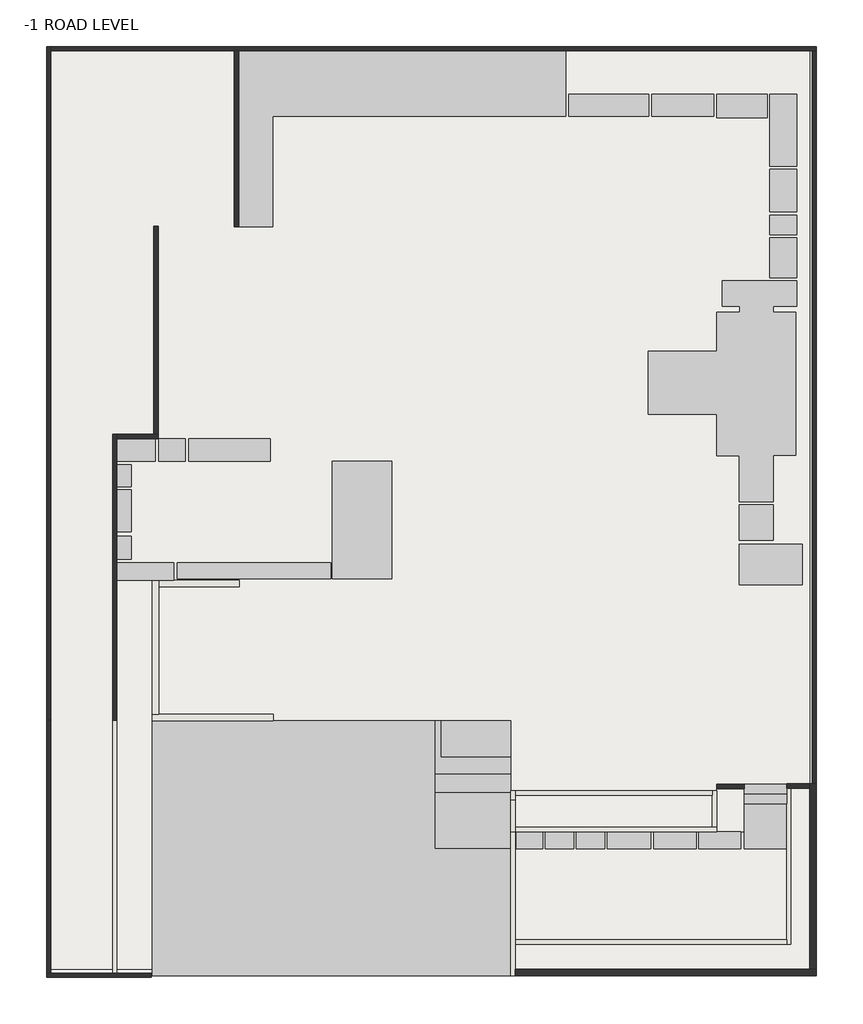
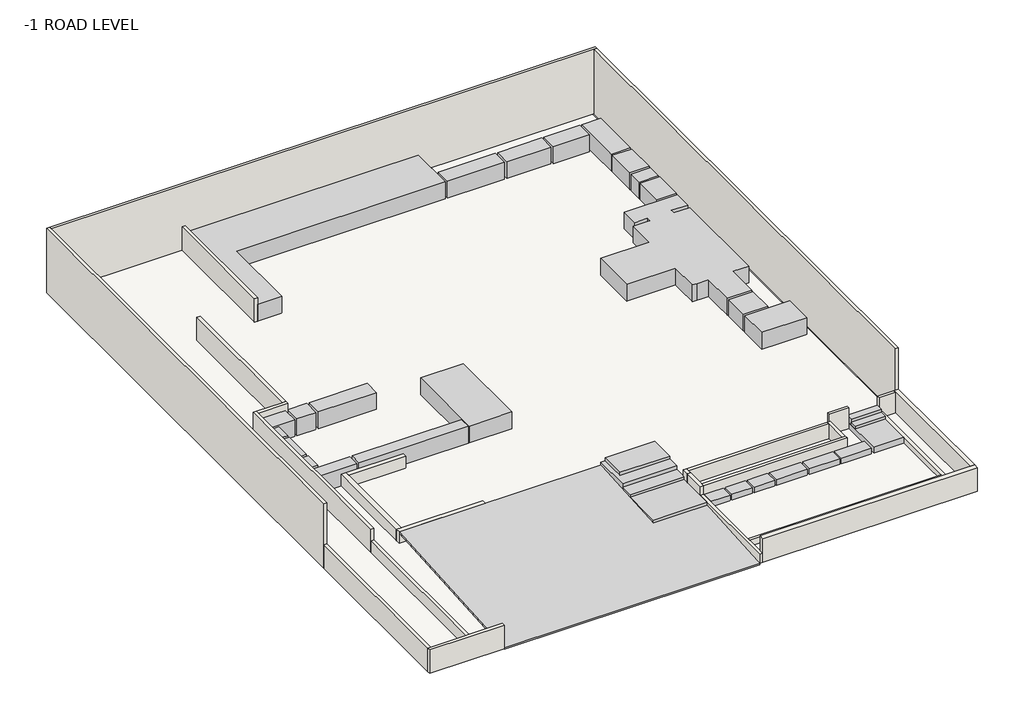
# One storey: 25 walls, 2 proxies, 2 slabs, 1 ramp.
"""IFC4 building model written with IfcOpenShell, lengths in millimetres."""

from ifc_helpers import new_model, si_unit, frame, origin, place, context, project, spatial, polyline, outline, extrude, faceted_brep, transform, mapped, element, save
from components import generic_models_1_generic_models_1_8db9de98, generic_models_2_generic_models_2_cbc3407a, ramp_2_3d1851f7

model = new_model("IFC4")

# Units and contexts
model_context = context("Model", 3, world=origin())
ifc_project = project(units=[si_unit("LENGTHUNIT", "METRE", prefix="MILLI")], contexts=[model_context])

# Site, building, storey
site = spatial("IfcSite", under=ifc_project)
building = spatial("IfcBuilding", under=site)
storey = spatial("IfcBuildingStorey", under=building, Name="-1 ROAD LEVEL", Elevation=-914.4)

# Proxies
placement = place(None, origin())
generic_models_1_generic_models_1_shape = generic_models_1_generic_models_1_8db9de98(model_context)
element("IfcBuildingElementProxy", 1, Name="Generic Models 1 : Generic Models 1", ObjectType="Generic Models 1 : Generic Models 1", at=placement, inside=storey, context=model_context, shape_type="MappedRepresentation", body=[
    mapped(generic_models_1_generic_models_1_shape, transform((0.0, 0.0, 0.0), x_axis=(1.0, 0.0, 0.0), y_axis=(0.0, 1.0, 0.0), z_axis=(0.0, 0.0, 1.0))),
])
generic_models_2_generic_models_2_shape = generic_models_2_generic_models_2_cbc3407a(model_context)
element("IfcBuildingElementProxy", 2, Name="Generic Models 2 : Generic Models 2", ObjectType="Generic Models 2 : Generic Models 2", at=placement, inside=storey, context=model_context, shape_type="MappedRepresentation", body=[
    mapped(generic_models_2_generic_models_2_shape, transform((0.0, 0.0, 0.0), x_axis=(1.0, 0.0, 0.0), y_axis=(0.0, 1.0, 0.0), z_axis=(0.0, 0.0, 1.0))),
])

# Ramp
ramp_2_shape = ramp_2_3d1851f7(model_context)
element("IfcRamp", 3, ObjectType="Ramp 2", at=placement, inside=storey, context=model_context, shape_type="MappedRepresentation", body=[
    mapped(ramp_2_shape, transform((0.0, 0.0, 0.0), x_axis=(1.0, 0.0, 0.0), y_axis=(0.0, 1.0, 0.0), z_axis=(0.0, 0.0, 1.0))),
])

# Slabs
element("IfcSlab", 4, ObjectType="6\"", at=placement, inside=storey, context=model_context, shape_type="SweptSolid", body=[
    extrude(outline(polyline([(7185.8179176, -9972.5794723), (7185.8179176, -11102.8794723), (282.0588295, -11102.8794723), (282.0588295, -9972.5794723), (7185.8179176, -9972.5794723)])), frame((0.0, 0.0, -914.4), z_axis=(0.0, 0.0, 1.0), x_axis=(1.0, 0.0, 0.0)), (0.0, 0.0, 1.0), 152.4),
    extrude(outline(polyline([(8295.7588295, -9743.9794723), (8295.7588295, -11255.2794723), (7338.2179176, -11255.2794723), (7338.2179176, -9743.9794723), (8295.7588295, -9743.9794723)])), frame((0.0, 0.0, -914.4), z_axis=(0.0, 0.0, 1.0), x_axis=(1.0, 0.0, 0.0)), (0.0, 0.0, 1.0), 152.4),
    extrude(outline(polyline([(10594.4588295, -9735.0018845), (10594.4588295, -16072.3018845), (9934.0588295, -16072.3018845), (282.0588295, -16072.3018845), (282.0588295, -15196.0018845), (9934.0588295, -15196.0018845), (9934.0588295, -9735.0018845), (10594.4588295, -9735.0018845)])), frame((0.0, 0.0, -914.4), z_axis=(0.0, 0.0, 1.0), x_axis=(1.0, 0.0, 0.0)), (0.0, 0.0, 1.0), 152.4),
    extrude(outline(polyline([(9781.6588295, -11267.9794723), (9781.6588295, -15043.6018845), (282.0588295, -15043.6018845), (282.0588295, -11267.9794723), (9781.6588295, -11267.9794723)])), frame((0.0, 0.0, -914.4), z_axis=(0.0, 0.0, 1.0), x_axis=(1.0, 0.0, 0.0)), (0.0, 0.0, 1.0), 152.4),
])
element("IfcSlab", 5, ObjectType="6\"", at=placement, inside=storey, context=model_context, shape_type="SweptSolid", body=[
    extrude(outline(polyline([(10594.4588295, 16064.6306443), (10594.4588295, -16072.3018845), (-15958.8181368, -16072.3018845), (-15958.8181368, 16064.6306443), (10594.4588295, 16064.6306443)])), frame((0.0, 0.0, -1066.8), z_axis=(0.0, 0.0, 1.0), x_axis=(1.0, 0.0, 0.0)), (0.0, 0.0, 1.0), 152.4),
])

# Walls
element("IfcWall", 6, ObjectType="6", at=placement, inside=storey, context=model_context, shape_type="Brep", body=[
    faceted_brep([(129.6588295, -10163.0794723, -914.4), (129.6588295, -11255.2794723, -914.4), (129.6588295, -11255.2794723, -457.2), (129.6588295, -11255.2794723, 0.0), (129.6588295, -10163.0794723, 0.0), (282.0588295, -10163.0794723, -914.4), (282.0588295, -10163.0794723, 0.0), (282.0588295, -11102.8794723, 0.0), (282.0588295, -11255.2794723, 0.0), (282.0588295, -11255.2794723, -457.2), (282.0588295, -11255.2794723, -914.4), (282.0588295, -11102.8794723, -914.4)], [[[0, 1, 2, 3, 4]], [[5, 6, 7, 8, 9, 10, 11]], [[1, 0, 5, 11, 10]], [[4, 3, 8, 7, 6]], [[0, 4, 6, 5]], [[1, 10, 9, 8, 3, 2]]]),
])
element("IfcWall", 7, ObjectType="6", at=placement, inside=storey, context=model_context, shape_type="Brep", body=[
    faceted_brep([(282.0588295, -11255.2794723, 0.0), (282.0588295, -11255.2794723, -914.4), (7338.2179176, -11255.2794723, -914.4), (7338.2179176, -11255.2794723, 0.0), (282.0588295, -11102.8794723, -914.4), (282.0588295, -11102.8794723, 0.0), (7185.8179176, -11102.8794723, 0.0), (7338.2179176, -11102.8794723, 0.0), (7338.2179176, -11102.8794723, -914.4), (7185.8179176, -11102.8794723, -914.4)], [[[0, 1, 2, 3]], [[4, 5, 6, 7, 8, 9]], [[2, 1, 4, 9, 8]], [[0, 3, 7, 6, 5]], [[3, 2, 8, 7]], [[0, 5, 4, 1]]]),
])
element("IfcWall", 8, ObjectType="6", at=placement, inside=storey, context=model_context, shape_type="Brep", body=[
    faceted_brep([(7338.2179176, -11102.8794723, -914.4), (7338.2179176, -9820.1794723, -914.4), (7338.2179176, -9820.1794723, 0.0), (7338.2179176, -11102.8794723, 0.0), (7185.8179176, -11102.8794723, -914.4), (7185.8179176, -11102.8794723, 0.0), (7185.8179176, -9972.5794723, 0.0), (7185.8179176, -9820.1794723, 0.0), (7185.8179176, -9820.1794723, -914.4), (7185.8179176, -9972.5794723, -914.4)], [[[0, 1, 2, 3]], [[4, 5, 6, 7, 8, 9]], [[1, 0, 4, 9, 8]], [[3, 2, 7, 6, 5]], [[0, 3, 5, 4]], [[2, 1, 8, 7]]]),
])
element("IfcWall", 9, ObjectType="6", at=placement, inside=storey, context=model_context, shape_type="SweptSolid", body=[
    extrude(outline(polyline([(282.0588295, -9820.1794723), (7185.8179176, -9820.1794723), (7185.8179176, -9972.5794723), (282.0588295, -9972.5794723), (282.0588295, -9820.1794723)])), frame((0.0, 0.0, -914.4), z_axis=(0.0, 0.0, 1.0), x_axis=(1.0, 0.0, 0.0)), (0.0, 0.0, 1.0), 914.4),
])
element("IfcWall", 10, ObjectType="6", at=placement, inside=storey, context=model_context, shape_type="Brep", body=[
    faceted_brep([(282.0588295, -10163.0794723, -914.4), (282.0588295, -9972.5794723, -914.4), (282.0588295, -9820.1794723, -914.4), (282.0588295, -9820.1794723, 0.0), (282.0588295, -9972.5794723, 0.0), (282.0588295, -10163.0794723, 0.0), (129.6588295, -10163.0794723, -914.4), (129.6588295, -10163.0794723, 0.0), (129.6588295, -9820.1794723, 0.0), (129.6588295, -9820.1794723, -914.4)], [[[0, 1, 2, 3, 4, 5]], [[6, 7, 8, 9]], [[2, 1, 0, 6, 9]], [[5, 4, 3, 8, 7]], [[0, 5, 7, 6]], [[3, 2, 9, 8]]]),
])
element("IfcWall", 11, ObjectType="6", at=placement, inside=storey, context=model_context, shape_type="Brep", body=[
    faceted_brep([(129.6588295, -11255.2794723, -914.4), (129.6588295, -16300.9018845, -914.4), (129.6588295, -16300.9018845, -457.2), (129.6588295, -11255.2794723, -457.2), (282.0588295, -11255.2794723, -914.4), (282.0588295, -11255.2794723, -457.2), (282.0588295, -15043.6018845, -457.2), (282.0588295, -15196.0018845, -457.2), (282.0588295, -16300.9018845, -457.2), (282.0588295, -16300.9018845, -914.4), (282.0588295, -16072.3018845, -914.4), (282.0588295, -15196.0018845, -914.4), (282.0588295, -15043.6018845, -914.4)], [[[0, 1, 2, 3]], [[4, 5, 6, 7, 8, 9, 10, 11, 12]], [[1, 0, 4, 12, 11, 10, 9]], [[3, 2, 8, 7, 6, 5]], [[0, 3, 5, 4]], [[2, 1, 9, 8]]]),
])
element("IfcWall", 12, ObjectType="6", at=placement, inside=storey, context=model_context, shape_type="Brep", body=[
    faceted_brep([(10594.4588295, -9582.6018845, -914.4), (9781.6588295, -9582.6018845, -914.4), (9781.6588295, -9582.6018845, 304.8), (10594.4588295, -9582.6018845, 304.8), (10594.4588295, -9735.0018845, -914.4), (10594.4588295, -9735.0018845, 304.8), (9781.6588295, -9735.0018845, 304.8), (9781.6588295, -9735.0018845, -457.2), (9781.6588295, -9735.0018845, -914.4), (9934.0588295, -9735.0018845, -914.4)], [[[0, 1, 2, 3]], [[4, 5, 6, 7, 8, 9]], [[1, 0, 4, 9, 8]], [[3, 2, 6, 5]], [[0, 3, 5, 4]], [[2, 1, 8, 7, 6]]]),
])
element("IfcWall", 13, ObjectType="6", at=placement, inside=storey, context=model_context, shape_type="Brep", body=[
    faceted_brep([(9781.6588295, -9735.0018845, -914.4), (9781.6588295, -15043.6018845, -914.4), (9781.6588295, -15196.0018845, -914.4), (9781.6588295, -15196.0018845, -457.2), (9781.6588295, -15043.6018845, -457.2), (9781.6588295, -9735.0018845, -457.2), (9934.0588295, -9735.0018845, -914.4), (9934.0588295, -9735.0018845, -457.2), (9934.0588295, -15196.0018845, -457.2), (9934.0588295, -15196.0018845, -914.4)], [[[0, 1, 2, 3, 4, 5]], [[6, 7, 8, 9]], [[2, 1, 0, 6, 9]], [[5, 4, 3, 8, 7]], [[0, 5, 7, 6]], [[3, 2, 9, 8]]]),
])
element("IfcWall", 14, ObjectType="6", at=placement, inside=storey, context=model_context, shape_type="SweptSolid", body=[
    extrude(outline(polyline([(282.0588295, -15043.6018845), (9781.6588295, -15043.6018845), (9781.6588295, -15196.0018845), (282.0588295, -15196.0018845), (282.0588295, -15043.6018845)])), frame((0.0, 0.0, -914.4), z_axis=(0.0, 0.0, 1.0), x_axis=(1.0, 0.0, 0.0)), (0.0, 0.0, 1.0), 457.2),
])
element("IfcWall", 15, ObjectType="6", at=placement, inside=storey, context=model_context, shape_type="Brep", body=[
    faceted_brep([(8295.7588295, -9591.5794723, -914.4), (7338.2179176, -9591.5794723, -914.4), (7338.2179176, -9591.5794723, 0.0), (7338.2179176, -9591.5794723, 304.8), (8295.7588295, -9591.5794723, 304.8), (8295.7588295, -9743.9794723, -914.4), (8295.7588295, -9743.9794723, 304.8), (7338.2179176, -9743.9794723, 304.8), (7338.2179176, -9743.9794723, -914.4)], [[[0, 1, 2, 3, 4]], [[5, 6, 7, 8]], [[1, 0, 5, 8]], [[4, 3, 7, 6]], [[0, 4, 6, 5]], [[3, 2, 1, 8, 7]]]),
])
element("IfcWall", 16, ObjectType="6", at=placement, inside=storey, context=model_context, shape_type="Brep", body=[
    faceted_brep([(-12453.6181368, -16202.8712384, -914.4), (-13647.4181368, -16202.8712384, -914.4), (-13799.8181368, -16202.8712384, -914.4), (-15958.8181368, -16202.8712384, -914.4), (-16111.2181368, -16202.8712384, -914.4), (-16111.2181368, -16202.8712384, 304.8), (-15958.8181368, -16202.8712384, 304.8), (-12453.6181368, -16202.8712384, 304.8), (-12453.6181368, -16355.2712384, -914.4), (-12453.6181368, -16355.2712384, 304.8), (-16111.2181368, -16355.2712384, 304.8), (-16111.2181368, -16355.2712384, -914.4)], [[[0, 1, 2, 3, 4, 5, 6, 7]], [[8, 9, 10, 11]], [[4, 3, 2, 1, 0, 8, 11]], [[7, 6, 5, 10, 9]], [[0, 7, 9, 8]], [[5, 4, 11, 10]]]),
])
element("IfcWall", 17, ObjectType="6", at=placement, inside=storey, context=model_context, shape_type="Brep", body=[
    faceted_brep([(-15958.8181368, 16064.6306443, -914.4), (-9546.1178012, 16064.6306443, -914.4), (-9393.7178012, 16064.6306443, -914.4), (10672.4840945, 16064.6306443, -914.4), (10824.8840945, 16064.6306443, -914.4), (10824.8840945, 16064.6306443, 2438.4), (10672.4840945, 16064.6306443, 2438.4), (-15958.8181368, 16064.6306443, 2438.4), (-15958.8181368, 16217.0306443, -914.4), (-15958.8181368, 16217.0306443, 2438.4), (10824.8840945, 16217.0306443, 2438.4), (10824.8840945, 16217.0306443, -914.4)], [[[0, 1, 2, 3, 4, 5, 6, 7]], [[8, 9, 10, 11]], [[4, 3, 2, 1, 0, 8, 11]], [[7, 6, 5, 10, 9]], [[5, 4, 11, 10]], [[0, 7, 9, 8]]]),
])
element("IfcWall", 18, ObjectType="6", at=placement, inside=storey, context=model_context, shape_type="Brep", body=[
    faceted_brep([(10672.4840945, 16064.6306443, -914.4), (10672.4840945, -9582.6018845, -914.4), (10672.4840945, -9582.6018845, 2438.4), (10672.4840945, 16064.6306443, 2438.4), (10824.8840945, 16064.6306443, -914.4), (10824.8840945, 16064.6306443, 2438.4), (10824.8840945, -9582.6018845, 2438.4), (10824.8840945, -9582.6018845, -914.4), (10823.0588295, -9582.6018845, -914.4)], [[[0, 1, 2, 3]], [[4, 5, 6, 7]], [[1, 0, 4, 7, 8]], [[3, 2, 6, 5]], [[0, 3, 5, 4]], [[2, 1, 8, 7, 6]]]),
])
element("IfcWall", 19, ObjectType="6", at=placement, inside=storey, context=model_context, shape_type="SweptSolid", body=[
    extrude(outline(polyline([(-15958.8181368, -7363.6712384), (-15958.8181368, -16202.8712384), (-16111.2181368, -16202.8712384), (-16111.2181368, -7363.6712384), (-15958.8181368, -7363.6712384)])), frame((0.0, 0.0, -914.4), z_axis=(0.0, 0.0, 1.0), x_axis=(1.0, 0.0, 0.0)), (0.0, 0.0, 1.0), 1219.2),
])
element("IfcWall", 20, ObjectType="6", at=placement, inside=storey, context=model_context, shape_type="Brep", body=[
    faceted_brep([(-15958.8181368, -7363.6712384, -914.4), (-15958.8181368, 16064.6306443, -914.4), (-15958.8181368, 16217.0306443, -914.4), (-15958.8181368, 16217.0306443, 2438.4), (-15958.8181368, 16064.6306443, 2438.4), (-15958.8181368, -7363.6712384, 2438.4), (-15958.8181368, -7363.6712384, 304.8), (-16111.2181368, -7363.6712384, -914.4), (-16111.2181368, -7363.6712384, 304.8), (-16111.2181368, -7363.6712384, 2438.4), (-16111.2181368, 16217.0306443, 2438.4), (-16111.2181368, 16217.0306443, -914.4)], [[[0, 1, 2, 3, 4, 5, 6]], [[7, 8, 9, 10, 11]], [[2, 1, 0, 7, 11]], [[5, 4, 3, 10, 9]], [[0, 6, 5, 9, 8, 7]], [[3, 2, 11, 10]]]),
])
element("IfcWall", 21, ObjectType="6", at=placement, inside=storey, context=model_context, shape_type="SweptSolid", body=[
    extrude(outline(polyline([(-13647.4181368, -7363.6712384), (-13647.4181368, -16202.8712384), (-13799.8181368, -16202.8712384), (-13799.8181368, -7363.6712384), (-13647.4181368, -7363.6712384)])), frame((0.0, 0.0, -914.4), z_axis=(0.0, 0.0, 1.0), x_axis=(1.0, 0.0, 0.0)), (0.0, 0.0, 1.0), 609.6),
])
element("IfcWall", 22, ObjectType="6", at=placement, inside=storey, context=model_context, shape_type="Brep", body=[
    faceted_brep([(-13647.4181368, 2491.5287616, -914.4), (-12199.6181368, 2491.5287616, -914.4), (-12199.6181368, 2491.5287616, 304.8), (-13647.4181368, 2491.5287616, 304.8), (-13647.4181368, 2643.9287616, -914.4), (-13647.4181368, 2643.9287616, 304.8), (-12352.0181368, 2643.9287616, 304.8), (-12199.6181368, 2643.9287616, 304.8), (-12199.6181368, 2643.9287616, -914.4), (-12352.0181368, 2643.9287616, -914.4)], [[[0, 1, 2, 3]], [[4, 5, 6, 7, 8, 9]], [[1, 0, 4, 9, 8]], [[3, 2, 7, 6, 5]], [[0, 3, 5, 4]], [[2, 1, 8, 7]]]),
])
element("IfcWall", 23, ObjectType="6", at=placement, inside=storey, context=model_context, shape_type="SweptSolid", body=[
    extrude(outline(polyline([(-12199.6181368, 9933.7287616), (-12199.6181368, 2643.9287616), (-12352.0181368, 2643.9287616), (-12352.0181368, 9933.7287616), (-12199.6181368, 9933.7287616)])), frame((0.0, 0.0, -914.4), z_axis=(0.0, 0.0, 1.0), x_axis=(1.0, 0.0, 0.0)), (0.0, 0.0, 1.0), 1219.2),
])
element("IfcWall", 24, ObjectType="6", at=placement, inside=storey, context=model_context, shape_type="Brep", body=[
    faceted_brep([(-13647.4181368, -7363.6712384, -914.4), (-13647.4181368, 2491.5287616, -914.4), (-13647.4181368, 2643.9287616, -914.4), (-13647.4181368, 2643.9287616, 304.8), (-13647.4181368, 2491.5287616, 304.8), (-13647.4181368, -7363.6712384, 304.8), (-13647.4181368, -7363.6712384, -304.8), (-13799.8181368, -7363.6712384, -914.4), (-13799.8181368, -7363.6712384, -304.8), (-13799.8181368, -7363.6712384, 304.8), (-13799.8181368, 2643.9287616, 304.8), (-13799.8181368, 2643.9287616, -914.4)], [[[0, 1, 2, 3, 4, 5, 6]], [[7, 8, 9, 10, 11]], [[2, 1, 0, 7, 11]], [[5, 4, 3, 10, 9]], [[0, 6, 5, 9, 8, 7]], [[3, 2, 11, 10]]]),
])
element("IfcWall", 25, ObjectType="6", at=placement, inside=storey, context=model_context, shape_type="SweptSolid", body=[
    extrude(outline(polyline([(-9393.7178012, 16064.6306443), (-9393.7178012, 9909.3951007), (-9546.1178012, 9909.3951007), (-9546.1178012, 16064.6306443), (-9393.7178012, 16064.6306443)])), frame((0.0, 0.0, -914.4), z_axis=(0.0, 0.0, 1.0), x_axis=(1.0, 0.0, 0.0)), (0.0, 0.0, 1.0), 1219.2),
])
element("IfcWall", 26, ObjectType="9", at=placement, inside=storey, context=model_context, shape_type="Brep", body=[
    faceted_brep([(282.0588295, -16300.9018845, -914.4), (10823.0588295, -16300.9018845, -914.4), (10823.0588295, -16300.9018845, 304.8), (282.0588295, -16300.9018845, 304.8), (282.0588295, -16300.9018845, -457.2), (282.0588295, -16072.3018845, -914.4), (282.0588295, -16072.3018845, 304.8), (10594.4588295, -16072.3018845, 304.8), (10823.0588295, -16072.3018845, 304.8), (10823.0588295, -16072.3018845, -914.4), (10594.4588295, -16072.3018845, -914.4)], [[[0, 1, 2, 3, 4]], [[5, 6, 7, 8, 9, 10]], [[1, 0, 5, 10, 9]], [[3, 2, 8, 7, 6]], [[0, 4, 3, 6, 5]], [[2, 1, 9, 8]]]),
])
element("IfcWall", 27, ObjectType="9", at=placement, inside=storey, context=model_context, shape_type="Brep", body=[
    faceted_brep([(10823.0588295, -16072.3018845, -914.4), (10823.0588295, -9582.6018845, -914.4), (10823.0588295, -9582.6018845, 304.8), (10823.0588295, -16072.3018845, 304.8), (10594.4588295, -16072.3018845, -914.4), (10594.4588295, -16072.3018845, 304.8), (10594.4588295, -9735.0018845, 304.8), (10594.4588295, -9582.6018845, 304.8), (10594.4588295, -9582.6018845, -914.4), (10594.4588295, -9735.0018845, -914.4), (10672.4840945, -9582.6018845, -914.4)], [[[0, 1, 2, 3]], [[4, 5, 6, 7, 8, 9]], [[1, 0, 4, 9, 8, 10]], [[3, 2, 7, 6, 5]], [[0, 3, 5, 4]], [[2, 1, 10, 8, 7]]]),
])
element("IfcWall", 28, ObjectType="9", at=placement, inside=storey, context=model_context, shape_type="Brep", body=[
    faceted_brep([(-8184.1001466, -7145.4266794, -914.4), (-12192.5789065, -7145.4266794, -914.4), (-12421.1789065, -7145.4266794, -914.4), (-12421.1789065, -7145.4266794, -304.8), (-12192.5789065, -7145.4266794, -304.8), (-8184.1001466, -7145.4266794, -304.8), (-8184.1001466, -7374.0266794, -914.4), (-8184.1001466, -7374.0266794, -304.8), (-12421.1789065, -7374.0266794, -304.8), (-12421.1789065, -7374.0266794, -914.4)], [[[0, 1, 2, 3, 4, 5]], [[6, 7, 8, 9]], [[2, 1, 0, 6, 9]], [[5, 4, 3, 8, 7]], [[0, 5, 7, 6]], [[3, 2, 9, 8]]]),
])
element("IfcWall", 29, ObjectType="9", at=placement, inside=storey, context=model_context, shape_type="Brep", body=[
    faceted_brep([(-12192.5789065, -7145.4266794, -914.4), (-12192.5789065, -2678.0731969, -914.4), (-12192.5789065, -2449.4731969, -914.4), (-12192.5789065, -2449.4731969, -304.8), (-12192.5789065, -2678.0731969, -304.8), (-12192.5789065, -7145.4266794, -304.8), (-12421.1789065, -7145.4266794, -914.4), (-12421.1789065, -7145.4266794, -304.8), (-12421.1789065, -2449.4731969, -304.8), (-12421.1789065, -2449.4731969, -914.4)], [[[0, 1, 2, 3, 4, 5]], [[6, 7, 8, 9]], [[2, 1, 0, 6, 9]], [[5, 4, 3, 8, 7]], [[0, 5, 7, 6]], [[3, 2, 9, 8]]]),
])
element("IfcWall", 30, ObjectType="9", at=placement, inside=storey, context=model_context, shape_type="SweptSolid", body=[
    extrude(outline(polyline([(-9373.1789065, -2678.0731969), (-12192.5789065, -2678.0731969), (-12192.5789065, -2449.4731969), (-9373.1789065, -2449.4731969), (-9373.1789065, -2678.0731969)])), frame((0.0, 0.0, -914.4), z_axis=(0.0, 0.0, 1.0), x_axis=(1.0, 0.0, 0.0)), (0.0, 0.0, 1.0), 609.6),
])

save(model, "model.ifc")

# Revit data of these elements
# Type "Ramp 2"
#   Assembly Code = "B1010600"
#   built-in parameter 1008304 = 0.25 (stored number, unit not read)
#   built-in parameter 1008303 = 30 (stored number, unit not read)
#   built-in parameter 1008301 = 12 (stored number, unit not read)
#   Function = 0
# Type "6\""
#   Assembly Code = "B1010"
#   Function = 0
#   Layers, outside or top first: 0' - 6" "Grass" (function 1)
# Type "6"
#   Assembly Code = "B2010"
#   Layers, outside or top first: 0' - 6" no material (function 1)
# Type "9"
#   Assembly Code = "B2010"
#   Layers, outside or top first: 0' - 9" no material (function 1)
# Element 1 (IfcBuildingElementProxy, "Generic Models 1 : Generic Models 1")
#   Phase Created = New Construction
# Element 2 (IfcBuildingElementProxy, "Generic Models 2 : Generic Models 2")
#   Phase Created = New Construction
# Element 3 (IfcRamp, "Ramp 2")
#   built-in parameter 1007275 = "DN"
#   built-in parameter 1007272 = "UP"
#   Width = 3' - 0"
#   built-in parameter 1007276 = 1
#   built-in parameter 1007274 = 1
#   built-in parameter 1007273 = 1
#   built-in parameter 1007271 = 1
#   Phase Created = New Construction
# Element 4 (IfcSlab, "6\"")
#   Height Offset From Level = 0' - 6"
#   Phase Created = New Construction
#   Materials on its faces: "Grass"
# Element 5 (IfcSlab, "6\"")
#   Height Offset From Level = 0' - 0"
#   Phase Created = New Construction
#   Materials on its faces: "Grass"
# Elements 6, 7, 8, 9, 10 (IfcWall, "6")
#   Top Offset = 0' - 0"
#   Base Offset = 0' - 0"
#   wall height = 3' - 0"
#   Phase Created = New Construction
#   Base Constraint = -1 ROAD LEVEL
#   Top Constraint = 1 PLINTH LEVEL
#   Materials on its faces: "Default Wall"
# Element 11 (IfcWall, "6")
#   Top Offset = -0' - 6"
#   Base Offset = 0' - 0"
#   wall height = 1' - 6"
#   Phase Created = New Construction
#   Base Constraint = -1 ROAD LEVEL
#   Top Constraint = 0 PARKING LEVEL
#   Materials on its faces: "Default Wall"
# Elements 12, 15, 16, 19, 22, 23, 24, 25 (IfcWall, "6")
#   Top Offset = 0' - 0"
#   Base Offset = 0' - 0"
#   Unconnected Height = 4' - 0"
#   wall height = 4' - 0"
#   Phase Created = New Construction
#   Base Constraint = -1 ROAD LEVEL
#   Materials on its faces: "Default Wall"
# Elements 13, 14 (IfcWall, "6")
#   Top Offset = 0' - 0"
#   Base Offset = 0' - 0"
#   Unconnected Height = 1' - 6"
#   wall height = 1' - 6"
#   Phase Created = New Construction
#   Base Constraint = -1 ROAD LEVEL
#   Materials on its faces: "Default Wall"
# Elements 17, 18, 20 (IfcWall, "6")
#   Top Offset = 0' - 0"
#   Base Offset = 0' - 0"
#   Unconnected Height = 11' - 0"
#   wall height = 11' - 0"
#   Phase Created = New Construction
#   Base Constraint = -1 ROAD LEVEL
#   Materials on its faces: "Default Wall"
# Element 21 (IfcWall, "6")
#   Top Offset = 0' - 0"
#   Base Offset = 0' - 0"
#   Unconnected Height = 2' - 0"
#   wall height = 2' - 0"
#   Phase Created = New Construction
#   Base Constraint = -1 ROAD LEVEL
#   Materials on its faces: "Default Wall"
# Elements 26, 27 (IfcWall, "9")
#   Top Offset = 0' - 0"
#   Base Offset = 0' - 0"
#   Unconnected Height = 4' - 0"
#   wall height = 4' - 0"
#   Phase Created = New Construction
#   Base Constraint = -1 ROAD LEVEL
#   Materials on its faces: "Default Wall"
# Elements 28, 29, 30 (IfcWall, "9")
#   Top Offset = 0' - 0"
#   Base Offset = 0' - 0"
#   Unconnected Height = 2' - 0"
#   wall height = 2' - 0"
#   Phase Created = New Construction
#   Base Constraint = -1 ROAD LEVEL
#   Materials on its faces: "Default Wall"
# Materials
#   "Grass": class "Generic", colour RGB 27 35 14, transparency 0, Description = "Physical material.", Cost = 0
#   "Default Wall": colour RGB 128 128 128, transparency 0, Cost = 0
